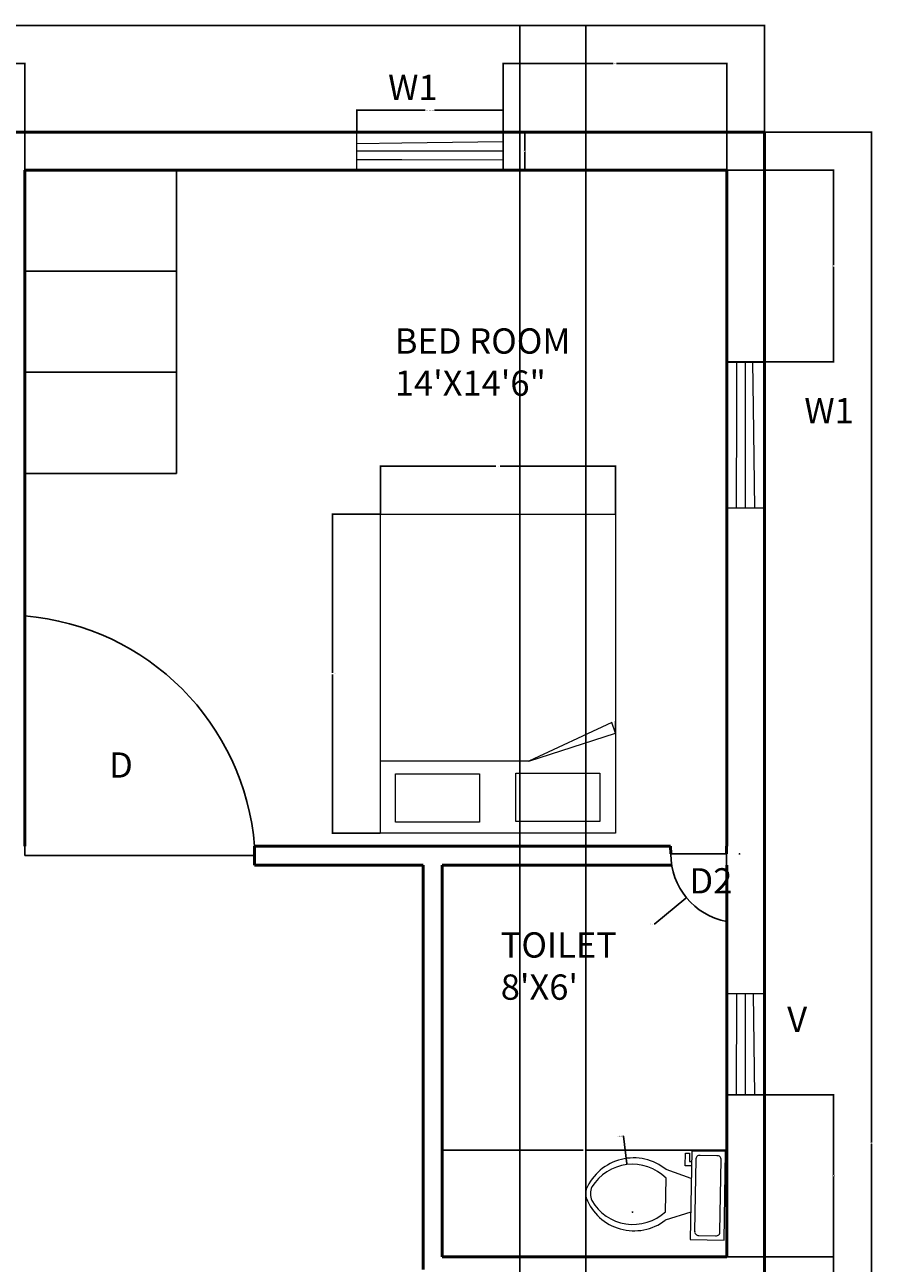
# Model space of a CAD drawing. Units: inches. Extents: x 2521 to 2933, y 1745 to 2276.
# Tile 4 of 4: x 2731 to 2933, y 1982 to 2276. Entities that reach past the tile are written whole.
import ezdxf

# ---------------------------------------------------------------- set-up
doc = ezdxf.new("R2010")
doc.units = ezdxf.units.IN
for name, color, linetype, lineweight in [('A-ANNO-DIMS', 2, 'Continuous', 18), ('A-ANNO-TEXT', 3, 'Continuous', 18), ('A-AREA-IDEN', 7, 'Continuous', 25), ('A-DOOR', 3, 'Continuous', 25), ('A-FLOR-CASE', 32, 'Continuous', 25), ('A-FLOR-FIXT', 9, 'Continuous', 18), ('A-FURN', 8, 'Continuous', 18), ('A-GLAZ', 4, 'Continuous', 20), ('A-WALL', 7, 'Continuous', 50)]:
    doc.layers.add(name, color=color, linetype=linetype, lineweight=lineweight)
doc.styles.get("Standard").update_dxf_attribs({"font": 'arial.ttf'})
doc.dimstyles.get("Standard").update_dxf_attribs({"dimtxt": 0.18, "dimasz": 0.18, "dimexe": 0.18, "dimexo": 0.0625, "dimgap": 0.09, "dimtad": 0, "dimtih": 1, "dimtoh": 1, "dimdec": 4, "dimzin": 0, "dimdsep": 46, "dimtxsty": 'Standard', "dimcen": 0.09, "dimadec": 0, "dimazin": 0, "dimtfac": 1, "dimtdec": 4, "dimtofl": 0, "dimtmove": 0, "dimatfit": 3, "dimfxl": 1, "dimtolj": 1, "dimtzin": 0, "dimarcsym": 0})

# ---------------------------------------------------------------- blocks, each defined once
blk = doc.blocks.new('Toilet - top')
for p, q in [((9.5, -6), (9.5, -2)), ((-10, -8.5), (-8, -8.5)), ((-10, -9.5), (-10, -8.5)), ((-8, -8.5), (-8, -8)), ((-7, -8), (-7, -9.5)), ((-4, -8), (-6, -14)), ((4, -8), (6, -14)), ((-7, -9.5), (-10, -9.5)), ((4, -14), (-4, -14))]:
    blk.add_line(p, q)
blk.add_lwpolyline([(10.5, -8), (10.5, 0), (-10.5, 0), (-10.5, -8)], close=True)
for points in [[(-9.5, -2), (-9.5, -6)], [(8.5, -1), (-8.5, -1)], [(-8.5, -7), (8.5, -7)]]:
    blk.add_lwpolyline(points)
for centre, radius, start, end in [((-8.62, -1.88), 0.884, 81.8699, 188.1301), ((8.62, -1.88), 0.884, 351.8699, 98.1301), ((-8.62, -6.12), 0.884, 171.8699, 278.1301), ((8.62, -6.12), 0.884, 261.8699, 8.1301), ((3.52, -21.58), 12.17, 141.4691, 247.9714), ((4.2, -21.82), 11.33, 136.3677, 238.9468), ((-3.52, -21.58), 12.17, 292.0284, 38.5307), ((-4.2, -21.82), 11.33, 301.053, 43.6321), ((0, -27.88), 4, 245.7318, 294.2682), ((0, -29), 4, 254.8605, 285.1395)]:
    blk.add_arc(centre, radius, start, end)
blk = doc.blocks.new('WINDOW-W1-LONG')
for p, q in [((0, 24), (0, 34.69)), ((0, 34.69), (9, 34.69)), ((2.4, 24), (2.44, 34.69)), ((4.5, 24), (4.5, 34.69)), ((6.37, 24), (6.23, 34.69)), ((9, 34.69), (9, 24)), ((0, 24), (0, 0)), ((2.32, 0), (2.4, 24)), ((4.5, 0), (4.5, 24)), ((6.68, 0), (6.37, 24)), ((9, 24), (9, 0)), ((9, 0), (0, 0))]:
    blk.add_line(p, q)
blk = doc.blocks.new('WINDOW-24')
for p, q in [((9, 24), (0, 24)), ((0, 24), (0, 0)), ((2.32, 0), (2.4, 24)), ((4.5, 0), (4.5, 24)), ((6.68, 0), (6.37, 24)), ((9, 24), (9, 0)), ((9, 0), (0, 0))]:
    blk.add_line(p, q)
blk = doc.blocks.new('DOOR-SINGLE-SWING')
for p, q in [((54.54, 0), (54.54, 56.86)), ((0, 0), (54.54, 0))]:
    blk.add_line(p, q)
blk.add_arc((59.46, -2.59), 59.65, 94.7338, 175.398)
blk = doc.blocks.new('BED-DOUBLE')
for p, q in [((55.72, 23.76), (55.72, 26.62)), ((54.9, 26.24), (35.19, 17.12)), ((35.19, 17.12), (55.72, 23.76)), ((55.72, 23.76), (54.9, 26.24)), ((35.19, 17.12), (0, 17.12))]:
    blk.add_line(p, q)
for points in [[(0, 75.73), (55.72, 75.73), (55.72, 0), (0, 0)], [(3.53, 14.11), (23.44, 14.11), (23.44, 2.6), (3.53, 2.6)], [(32.11, 14.25), (52.02, 14.25), (52.02, 2.74), (32.11, 2.74)]]:
    blk.add_lwpolyline(points, close=True)
blk = doc.blocks.new('CABINET-3-BAY')
for p, q in [((0, 0), (0, 72)), ((0, 48), (36, 48)), ((0, 24), (36, 24)), ((0, 0), (36, 0))]:
    blk.add_line(p, q)
blk = doc.blocks.new('*D9')
at = {"layer": 'A-ANNO-DIMS', "color": 0, "lineweight": -2, "transparency": 16777216}
for p, q in [((2810.24, 2250.34), (2810.24, 2255.67)), ((2810.42, 2255.49), (2826.47, 2255.49)), ((2844.76, 2255.49), (2828.71, 2255.49)), ((2844.94, 2250.34), (2844.94, 2255.67))]:
    blk.add_line(p, q, dxfattribs=at)
at = {"layer": 'A-ANNO-DIMS', "color": 0, "transparency": 16777216}
for points in [[(2810.42, 2255.52), (2810.42, 2255.46), (2810.24, 2255.49)], [(2844.76, 2255.52), (2844.76, 2255.46), (2844.94, 2255.49)]]:
    blk.add_solid(points, dxfattribs=at)
at = {"layer": 'Defpoints', "color": 0, "transparency": 16777216}
for p in [(2810.24, 2255.49), (2810.24, 2250.28), (2844.94, 2250.28)]:
    blk.add_point(p, dxfattribs=at)
at = {"layer": 'A-ANNO-DIMS', "color": 0, "transparency": 16777216, "insert": (2827.59, 2255.49), "char_height": 0.18, "attachment_point": 5}
blk.add_mtext('\\A1;WINDOW 35 TYP.', dxfattribs=at)
blk = doc.blocks.new('*D10')
at = {"layer": 'A-ANNO-DIMS', "color": 0, "lineweight": -2, "transparency": 16777216}
for p, q in [((2845, 2250.28), (2850.32, 2250.28)), ((2850.14, 2250.1), (2850.14, 2245.96)), ((2850.14, 2241.46), (2850.14, 2245.6)), ((2845, 2241.28), (2850.32, 2241.28))]:
    blk.add_line(p, q, dxfattribs=at)
at = {"layer": 'A-ANNO-DIMS', "color": 0, "transparency": 16777216}
for points in [[(2850.11, 2250.1), (2850.17, 2250.1), (2850.14, 2250.28)], [(2850.11, 2241.46), (2850.17, 2241.46), (2850.14, 2241.28)]]:
    blk.add_solid(points, dxfattribs=at)
at = {"layer": 'Defpoints', "color": 0, "transparency": 16777216}
for p in [(2844.94, 2250.28), (2850.14, 2250.28), (2844.94, 2241.28)]:
    blk.add_point(p, dxfattribs=at)
at = {"layer": 'A-ANNO-DIMS', "color": 0, "transparency": 16777216, "insert": (2850.14, 2245.78), "char_height": 0.18, "attachment_point": 5}
blk.add_mtext('\\A1;9 TYP.', dxfattribs=at)
blk = doc.blocks.new('*D13')
at = {"layer": 'A-ANNO-DIMS', "color": 0, "lineweight": -2, "transparency": 16777216}
for p, q in [((2815.82, 2159.61), (2804.34, 2159.61)), ((2804.52, 2159.43), (2804.52, 2121.93)), ((2804.52, 2084.06), (2804.52, 2121.56)), ((2815.82, 2083.88), (2804.34, 2083.88))]:
    blk.add_line(p, q, dxfattribs=at)
at = {"layer": 'A-ANNO-DIMS', "color": 0, "transparency": 16777216}
for points in [[(2804.49, 2159.43), (2804.55, 2159.43), (2804.52, 2159.61)], [(2804.49, 2084.06), (2804.55, 2084.06), (2804.52, 2083.88)]]:
    blk.add_solid(points, dxfattribs=at)
at = {"layer": 'Defpoints', "color": 0, "transparency": 16777216}
for p in [(2804.52, 2159.61), (2815.88, 2159.61), (2815.88, 2083.88)]:
    blk.add_point(p, dxfattribs=at)
at = {"layer": 'A-ANNO-DIMS', "color": 0, "transparency": 16777216, "insert": (2804.52, 2121.74), "char_height": 0.18, "attachment_point": 5}
blk.add_mtext('\\A1;BED 76 TYP.', dxfattribs=at)
blk = doc.blocks.new('*D14')
at = {"layer": 'A-ANNO-DIMS', "color": 0, "lineweight": -2, "transparency": 16777216}
for p, q in [((2815.88, 2159.67), (2815.88, 2171.15)), ((2816.06, 2170.97), (2843.21, 2170.97)), ((2871.42, 2170.97), (2844.27, 2170.97)), ((2871.6, 2159.67), (2871.6, 2171.15))]:
    blk.add_line(p, q, dxfattribs=at)
at = {"layer": 'A-ANNO-DIMS', "color": 0, "transparency": 16777216}
for points in [[(2816.06, 2171), (2816.06, 2170.94), (2815.88, 2170.97)], [(2871.42, 2171), (2871.42, 2170.94), (2871.6, 2170.97)]]:
    blk.add_solid(points, dxfattribs=at)
at = {"layer": 'Defpoints', "color": 0, "transparency": 16777216}
for p in [(2871.6, 2170.97), (2815.88, 2159.61), (2871.6, 2159.61)]:
    blk.add_point(p, dxfattribs=at)
at = {"layer": 'A-ANNO-DIMS', "color": 0, "transparency": 16777216, "insert": (2843.74, 2170.97), "char_height": 0.18, "attachment_point": 5}
blk.add_mtext('\\A1;56 TYP.', dxfattribs=at)
blk = doc.blocks.new('*D23')
at = {"layer": 'A-ANNO-DIMS', "color": 0, "lineweight": -2, "transparency": 16777216}
for p, q in [((2547.01, 2250.34), (2547.01, 2275.78)), ((2547.19, 2275.6), (2726.72, 2275.6)), ((2906.83, 2275.6), (2727.3, 2275.6)), ((2907.01, 2250.34), (2907.01, 2275.78))]:
    blk.add_line(p, q, dxfattribs=at)
at = {"layer": 'A-ANNO-DIMS', "color": 0, "transparency": 16777216}
for points in [[(2547.19, 2275.63), (2547.19, 2275.57), (2547.01, 2275.6)], [(2906.83, 2275.63), (2906.83, 2275.57), (2907.01, 2275.6)]]:
    blk.add_solid(points, dxfattribs=at)
at = {"layer": 'Defpoints', "color": 0, "transparency": 16777216}
for p in [(2907.01, 2275.6), (2547.01, 2250.28), (2907.01, 2250.28)]:
    blk.add_point(p, dxfattribs=at)
at = {"layer": 'A-ANNO-DIMS', "color": 0, "transparency": 16777216, "insert": (2727.01, 2275.6), "char_height": 0.18, "attachment_point": 5}
blk.add_mtext('\\A1;360', dxfattribs=at)
blk = doc.blocks.new('*D24')
at = {"layer": 'A-ANNO-DIMS', "color": 0, "lineweight": -2, "transparency": 16777216}
for p, q in [((2907.07, 2250.28), (2932.51, 2250.28)), ((2932.33, 2250.1), (2932.33, 2010.46)), ((2932.33, 1770.46), (2932.33, 2010.1)), ((2907.07, 1770.28), (2932.51, 1770.28))]:
    blk.add_line(p, q, dxfattribs=at)
at = {"layer": 'A-ANNO-DIMS', "color": 0, "transparency": 16777216}
for points in [[(2932.3, 2250.1), (2932.36, 2250.1), (2932.33, 2250.28)], [(2932.3, 1770.46), (2932.36, 1770.46), (2932.33, 1770.28)]]:
    blk.add_solid(points, dxfattribs=at)
at = {"layer": 'Defpoints', "color": 0, "transparency": 16777216}
for p in [(2907.01, 2250.28), (2932.33, 2250.28), (2907.01, 1770.28)]:
    blk.add_point(p, dxfattribs=at)
at = {"layer": 'A-ANNO-DIMS', "color": 0, "transparency": 16777216, "insert": (2932.33, 2010.28), "char_height": 0.18, "attachment_point": 5}
blk.add_mtext('\\A1;480', dxfattribs=at)
blk = doc.blocks.new('*D27')
at = {"layer": 'A-ANNO-DIMS', "color": 0, "lineweight": -2, "transparency": 16777216}
for p, q in [((2722.51, 2241.34), (2722.51, 2266.78)), ((2731.51, 2241.34), (2731.51, 2266.78)), ((2722.69, 2266.6), (2726.86, 2266.6)), ((2731.33, 2266.6), (2727.16, 2266.6))]:
    blk.add_line(p, q, dxfattribs=at)
at = {"layer": 'A-ANNO-DIMS', "color": 0, "transparency": 16777216}
for points in [[(2722.69, 2266.63), (2722.69, 2266.57), (2722.51, 2266.6)], [(2731.33, 2266.63), (2731.33, 2266.57), (2731.51, 2266.6)]]:
    blk.add_solid(points, dxfattribs=at)
at = {"layer": 'Defpoints', "color": 0, "transparency": 16777216}
for p in [(2731.51, 2266.6), (2722.51, 2241.28), (2731.51, 2241.28)]:
    blk.add_point(p, dxfattribs=at)
at = {"layer": 'A-ANNO-DIMS', "color": 0, "transparency": 16777216, "insert": (2727.01, 2266.6), "char_height": 0.18, "attachment_point": 5}
blk.add_mtext('\\A1;9', dxfattribs=at)
blk = doc.blocks.new('*D28')
at = {"layer": 'A-ANNO-DIMS', "color": 0, "lineweight": -2, "transparency": 16777216}
for p, q in [((2844.94, 2241.34), (2844.94, 2266.78)), ((2898.01, 2241.34), (2898.01, 2266.78)), ((2845.12, 2266.6), (2871.08, 2266.6)), ((2897.83, 2266.6), (2871.87, 2266.6))]:
    blk.add_line(p, q, dxfattribs=at)
at = {"layer": 'A-ANNO-DIMS', "color": 0, "transparency": 16777216}
for points in [[(2845.12, 2266.63), (2845.12, 2266.57), (2844.94, 2266.6)], [(2897.83, 2266.63), (2897.83, 2266.57), (2898.01, 2266.6)]]:
    blk.add_solid(points, dxfattribs=at)
at = {"layer": 'Defpoints', "color": 0, "transparency": 16777216}
for p in [(2898.01, 2266.6), (2844.94, 2241.28), (2898.01, 2241.28)]:
    blk.add_point(p, dxfattribs=at)
at = {"layer": 'A-ANNO-DIMS', "color": 0, "transparency": 16777216, "insert": (2871.47, 2266.6), "char_height": 0.18, "attachment_point": 5}
blk.add_mtext('\\A1;53.07', dxfattribs=at)
blk = doc.blocks.new('*D36')
at = {"layer": 'A-ANNO-DIMS', "color": 0, "lineweight": -2, "transparency": 16777216}
for p, q in [((2898.07, 1983.28), (2923.51, 1983.28)), ((2923.33, 1983.1), (2923.33, 1960.51)), ((2923.33, 1937.55), (2923.33, 1960.14)), ((2898.07, 1937.37), (2923.51, 1937.37))]:
    blk.add_line(p, q, dxfattribs=at)
at = {"layer": 'A-ANNO-DIMS', "color": 0, "transparency": 16777216}
for points in [[(2923.3, 1983.1), (2923.36, 1983.1), (2923.33, 1983.28)], [(2923.3, 1937.55), (2923.36, 1937.55), (2923.33, 1937.37)]]:
    blk.add_solid(points, dxfattribs=at)
at = {"layer": 'Defpoints', "color": 0, "transparency": 16777216}
for p in [(2898.01, 1983.28), (2898.01, 1937.37), (2923.33, 1937.37)]:
    blk.add_point(p, dxfattribs=at)
at = {"layer": 'A-ANNO-DIMS', "color": 0, "transparency": 16777216, "insert": (2923.33, 1960.32), "char_height": 0.18, "attachment_point": 5}
blk.add_mtext('\\A1;45.91', dxfattribs=at)
blk = doc.blocks.new('*D37')
at = {"layer": 'A-ANNO-DIMS', "color": 0, "lineweight": -2, "transparency": 16777216}
for p, q in [((2898.07, 2021.77), (2923.51, 2021.77)), ((2923.33, 2021.59), (2923.33, 2002.71)), ((2923.33, 1983.46), (2923.33, 2002.34)), ((2898.07, 1983.28), (2923.51, 1983.28))]:
    blk.add_line(p, q, dxfattribs=at)
at = {"layer": 'A-ANNO-DIMS', "color": 0, "transparency": 16777216}
for points in [[(2923.3, 2021.59), (2923.36, 2021.59), (2923.33, 2021.77)], [(2923.3, 1983.46), (2923.36, 1983.46), (2923.33, 1983.28)]]:
    blk.add_solid(points, dxfattribs=at)
at = {"layer": 'Defpoints', "color": 0, "transparency": 16777216}
for p in [(2898.01, 2021.77), (2898.01, 1983.28), (2923.33, 1983.28)]:
    blk.add_point(p, dxfattribs=at)
at = {"layer": 'A-ANNO-DIMS', "color": 0, "transparency": 16777216, "insert": (2923.33, 2002.52), "char_height": 0.18, "attachment_point": 5}
blk.add_mtext('\\A1;38.485', dxfattribs=at)
blk = doc.blocks.new('*D38')
at = {"layer": 'A-ANNO-DIMS', "color": 0, "lineweight": -2, "transparency": 16777216}
for p, q in [((2898.07, 2241.28), (2923.51, 2241.28)), ((2923.33, 2241.1), (2923.33, 2218.69)), ((2923.33, 2195.91), (2923.33, 2218.32)), ((2898.07, 2195.73), (2923.51, 2195.73))]:
    blk.add_line(p, q, dxfattribs=at)
at = {"layer": 'A-ANNO-DIMS', "color": 0, "transparency": 16777216}
for points in [[(2923.3, 2241.1), (2923.36, 2241.1), (2923.33, 2241.28)], [(2923.3, 2195.91), (2923.36, 2195.91), (2923.33, 2195.73)]]:
    blk.add_solid(points, dxfattribs=at)
at = {"layer": 'Defpoints', "color": 0, "transparency": 16777216}
for p in [(2898.01, 2241.28), (2898.01, 2195.73), (2923.33, 2195.73)]:
    blk.add_point(p, dxfattribs=at)
at = {"layer": 'A-ANNO-DIMS', "color": 0, "transparency": 16777216, "insert": (2923.33, 2218.5), "char_height": 0.18, "attachment_point": 5}
blk.add_mtext('\\A1;45.56', dxfattribs=at)
blk = doc.blocks.new('*D49')
at = {"layer": 'A-ANNO-DIMS', "color": 0, "lineweight": -2, "transparency": 16777216}
for p, q in [((2830.51, 1983.34), (2830.51, 2008.78)), ((2830.69, 2008.6), (2863.93, 2008.6)), ((2897.83, 2008.6), (2864.58, 2008.6)), ((2898.01, 1983.34), (2898.01, 2008.78))]:
    blk.add_line(p, q, dxfattribs=at)
at = {"layer": 'A-ANNO-DIMS', "color": 0, "transparency": 16777216}
for points in [[(2830.69, 2008.63), (2830.69, 2008.57), (2830.51, 2008.6)], [(2897.83, 2008.63), (2897.83, 2008.57), (2898.01, 2008.6)]]:
    blk.add_solid(points, dxfattribs=at)
at = {"layer": 'Defpoints', "color": 0, "transparency": 16777216}
for p in [(2898.01, 2008.6), (2830.51, 1983.28), (2898.01, 1983.28)]:
    blk.add_point(p, dxfattribs=at)
at = {"layer": 'A-ANNO-DIMS', "color": 0, "transparency": 16777216, "insert": (2864.26, 2008.6), "char_height": 0.18, "attachment_point": 5}
blk.add_mtext('\\A1;67.5', dxfattribs=at)
blk = doc.blocks.new('*D59')
at = {"layer": 'A-ANNO-DIMS', "color": 0, "lineweight": -2, "transparency": 16777216}
for p, q in [((2848.92, 1927.91), (2848.92, 2275.78)), ((2849.1, 2275.6), (2856.29, 2275.6)), ((2864.39, 2275.6), (2857.2, 2275.6)), ((2864.57, 1950.23), (2864.57, 2275.78))]:
    blk.add_line(p, q, dxfattribs=at)
at = {"layer": 'A-ANNO-DIMS', "color": 0, "transparency": 16777216}
for points in [[(2849.1, 2275.63), (2849.1, 2275.57), (2848.92, 2275.6)], [(2864.39, 2275.63), (2864.39, 2275.57), (2864.57, 2275.6)]]:
    blk.add_solid(points, dxfattribs=at)
at = {"layer": 'Defpoints', "color": 0, "transparency": 16777216}
for p in [(2864.57, 2275.6), (2864.57, 1950.17), (2848.92, 1927.85)]:
    blk.add_point(p, dxfattribs=at)
at = {"layer": 'A-ANNO-DIMS', "color": 0, "transparency": 16777216, "insert": (2856.74, 2275.6), "char_height": 0.18, "attachment_point": 5}
blk.add_mtext('\\A1;15.656', dxfattribs=at)
blk = doc.blocks.new('*D62')
at = {"layer": 'A-ANNO-DIMS', "color": 0, "lineweight": -2, "transparency": 16777216}
for p, q in [((2900.94, 2078.93), (2901.12, 2078.93)), ((2901.03, 2078.84), (2901.03, 2079.02)), ((2880.95, 2062.32), (2888.35, 2068.43)), ((2880.77, 2062.32), (2880.95, 2062.32))]:
    blk.add_line(p, q, dxfattribs=at)
at = {"layer": 'A-ANNO-DIMS', "color": 0, "transparency": 16777216}
blk.add_solid([(2888.33, 2068.45), (2888.36, 2068.41), (2888.48, 2068.55)], dxfattribs=at)
at = {"layer": 'Defpoints', "color": 0, "transparency": 16777216}
for p in [(2901.03, 2078.93), (2888.48, 2068.55)]:
    blk.add_point(p, dxfattribs=at)
at = {"layer": 'A-ANNO-DIMS', "color": 0, "transparency": 16777216, "insert": (2880.23, 2062.32), "char_height": 0.18, "attachment_point": 5}
blk.add_mtext('\\A1;R16.286', dxfattribs=at)
blk = doc.blocks.new('*D65')
at = {"layer": 'A-ANNO-DIMS', "color": 0, "lineweight": -2, "transparency": 16777216}
for p, q in [((2873.36, 2011.94), (2873.54, 2011.94)), ((2873.54, 2011.94), (2874.32, 2005.37)), ((2875.57, 1993.94), (2875.75, 1993.94)), ((2875.66, 1993.85), (2875.66, 1994.03))]:
    blk.add_line(p, q, dxfattribs=at)
at = {"layer": 'A-ANNO-DIMS', "color": 0, "transparency": 16777216}
blk.add_solid([(2874.35, 2005.37), (2874.29, 2005.36), (2874.34, 2005.19)], dxfattribs=at)
at = {"layer": 'Defpoints', "color": 0, "transparency": 16777216}
for p in [(2874.34, 2005.19), (2875.66, 1993.94)]:
    blk.add_point(p, dxfattribs=at)
at = {"layer": 'A-ANNO-DIMS', "color": 0, "transparency": 16777216, "insert": (2872.69, 2011.94), "char_height": 0.18, "attachment_point": 5}
blk.add_mtext('\\A1;4X R11.33', dxfattribs=at)

msp = doc.modelspace()

# ---------------------------------------------------------------- linework, layer by layer
at = {"layer": 'A-DOOR'}
for p, q in [((2884.7464, 2078.9456), (2898.0014, 2078.9456)), ((2898.0014, 2078.9456), (2898.0014, 2062.9248))]:
    msp.add_line(p, q, dxfattribs=at)
msp.add_arc((2901.0328, 2078.9266), 16.2864, 179.93294, 259.273035, dxfattribs=at)
at = {"layer": 'A-WALL'}
for p, q in [((2547.009, 2250.2819), (2907.009, 2250.2819)), ((2907.009, 2250.2819), (2907.009, 1770.2819)), ((2731.509, 2080.7819), (2731.509, 2241.2819)), ((2731.509, 2241.2819), (2898.009, 2241.2819)), ((2898.009, 2241.2819), (2898.009, 2080.7819)), ((2786.0146, 2080.7819), (2786.0146, 2078.585)), ((2884.7023, 2080.7819), (2786.0146, 2080.7819)), ((2786.0146, 2078.585), (2786.0146, 2076.2819)), ((2884.7464, 2078.9456), (2884.7023, 2080.7819)), ((2898.009, 2080.7819), (2898.0014, 2080.7819)), ((2898.0014, 2078.9456), (2898.0014, 2080.7819)), ((2786.0146, 2076.2819), (2826.009, 2076.2819)), ((2826.009, 1980.2819), (2826.009, 2076.2819)), ((2830.509, 1983.2819), (2830.509, 2076.2819)), ((2884.9625, 2076.2819), (2830.509, 2076.2819)), ((2898.009, 2076.2819), (2898.0014, 2076.2819)), ((2898.009, 2076.2819), (2898.009, 1983.2819)), ((2830.509, 1983.2819), (2898.009, 1983.2819))]:
    msp.add_line(p, q, dxfattribs=at)

# ---------------------------------------------------------------- block references
at = {"layer": 'A-DOOR', "extrusion": (0, 0, -1), "zscale": -1}
msp.add_blockref('DOOR-SINGLE-SWING', (-2786.0151, 2078.585), dxfattribs=at)
at = {"layer": 'A-FLOR-CASE', "extrusion": (0, 0, -1), "zscale": -1}
msp.add_blockref('CABINET-3-BAY', (-2767.5091, 2169.282), dxfattribs=at)
at = {"layer": 'A-FLOR-FIXT', "rotation": 269.0579063208954}
msp.add_blockref('Toilet - top', (2897.5453, 1997.7762), dxfattribs=at)
at = {"layer": 'A-FURN'}
msp.add_blockref('BED-DOUBLE', (2815.8826, 2083.8816), dxfattribs=at)
at = {"layer": 'A-GLAZ', "rotation": 89.99999999999766}
msp.add_blockref('WINDOW-W1-LONG', (2844.9366, 2241.2819), dxfattribs=at)
at = {"layer": 'A-GLAZ'}
for name, p in [('WINDOW-W1-LONG', (2898.009, 2161.0317)), ('WINDOW-24', (2898.009, 2021.7669))]:
    msp.add_blockref(name, p, dxfattribs=at)

# ---------------------------------------------------------------- texts
at = {"layer": 'A-ANNO-TEXT', "char_height": 6, "attachment_point": 1}
for s, width, insert in [('W1', 10.814281, (2817.6837, 2263.9193)), ('W1', 10.559342, (2916.4285, 2187.1685)), ('D', 11.775491, (2751.4953, 2103.0512)), ('D2', 4.490782, (2889.1703, 2075.5606)), ('V', 11.777725, (2912.3704, 2042.6568))]:
    msp.add_mtext_dynamic_manual_height_columns(s, width=width, gutter_width=5.8967, heights=[0], dxfattribs=dict(at, insert=insert))
at = {"layer": 'A-AREA-IDEN', "char_height": 6, "attachment_point": 1}
for s, width, insert in [('BED ROOM \\P14\'X14\'6"', 50.277821, (2819.2707, 2203.7086)), ("TOILET\\P8'X6'", 38.619361, (2844.4003, 2060.3331))]:
    msp.add_mtext_dynamic_manual_height_columns(s, width=width, gutter_width=5.8967, heights=[0], dxfattribs=dict(at, insert=insert))

# ---------------------------------------------------------------- dimensions: what is measured, and where the dimension line sits
at = {"layer": 'A-ANNO-DIMS'}
for base, p1, p2, override, picture, middle in [((2907.009, 2275.6019), (2547.009, 2250.2819), (2907.009, 2250.2819), {"dimdec": 0, "dimlfac": 1, "dimrnd": 0, "dimzin": 0, "dimdsep": 46, "dimlunit": 2}, '*D23', (2727.009, 2275.6019)), ((2864.5724, 2275.6019), (2848.9165, 1927.8472), (2864.5724, 1950.1723), {"dimdec": 3, "dimlfac": 1, "dimrnd": 0, "dimzin": 0, "dimdsep": 46, "dimlunit": 2}, '*D59', (2856.7445, 2275.6019)), ((2731.509, 2266.6019), (2722.509, 2241.2819), (2731.509, 2241.2819), {"dimdec": 0, "dimlfac": 1, "dimrnd": 0, "dimzin": 0, "dimdsep": 46, "dimlunit": 2}, '*D27', (2727.009, 2266.6019)), ((2898.009, 2266.6019), (2844.9364, 2241.2819), (2898.009, 2241.2819), {"dimdec": 2, "dimlfac": 1, "dimrnd": 0, "dimzin": 0, "dimdsep": 46, "dimlunit": 2}, '*D28', (2871.4727, 2266.6019)), ((2898.009, 2008.6019), (2830.509, 1983.2819), (2898.009, 1983.2819), {"dimdec": 1, "dimlfac": 1, "dimrnd": 0, "dimzin": 0, "dimdsep": 46, "dimlunit": 2}, '*D49', (2864.259, 2008.6019))]:
    dim = msp.add_linear_dim(base=base, p1=p1, p2=p2, dimstyle='Standard', override=override, dxfattribs=at)
    dim.commit()
    dim.dimension.update_dxf_attribs({"geometry": picture, "text_midpoint": middle})
for base, p1, p2, angle, text, picture, middle in [((2810.2421, 2255.486), (2844.9364, 2250.2819), (2810.2421, 2250.2819), 180, 'WINDOW <> TYP.', '*D9', (2827.5892, 2255.486)), ((2850.1405, 2250.2819), (2844.9364, 2241.2819), (2844.9364, 2250.2819), 90, '<> TYP.', '*D10', (2850.1405, 2245.7819)), ((2804.5236, 2159.608), (2815.8825, 2083.8819), (2815.8825, 2159.608), 90, 'BED <> TYP.', '*D13', (2804.5236, 2121.7449))]:
    dim = msp.add_linear_dim(base=base, p1=p1, p2=p2, angle=angle, text=text, dimstyle='Standard', override={"dimdec": 0, "dimlfac": 1, "dimrnd": 0, "dimzin": 0, "dimdsep": 46, "dimlunit": 2}, dxfattribs=at)
    dim.commit()
    dim.dimension.update_dxf_attribs({"geometry": picture, "text_midpoint": middle})
for base, p1, p2, angle, override, picture, middle in [((2932.329, 2250.2819), (2907.009, 1770.2819), (2907.009, 2250.2819), 90, {"dimdec": 0, "dimlfac": 1, "dimrnd": 0, "dimzin": 0, "dimdsep": 46, "dimlunit": 2}, '*D24', (2932.329, 2010.2819)), ((2923.329, 2195.7261), (2898.009, 2241.2819), (2898.009, 2195.7261), 270, {"dimdec": 2, "dimlfac": 1, "dimrnd": 0, "dimzin": 0, "dimdsep": 46, "dimlunit": 2}, '*D38', (2923.329, 2218.504)), ((2923.329, 1983.2819), (2898.009, 2021.7666), (2898.009, 1983.2819), 270, {"dimdec": 3, "dimlfac": 1, "dimrnd": 0, "dimzin": 0, "dimdsep": 46, "dimlunit": 2}, '*D37', (2923.329, 2002.5243)), ((2923.329, 1937.3677), (2898.009, 1983.2819), (2898.009, 1937.3677), 270, {"dimdec": 2, "dimlfac": 1, "dimrnd": 0, "dimzin": 0, "dimdsep": 46, "dimlunit": 2}, '*D36', (2923.329, 1960.3248))]:
    dim = msp.add_linear_dim(base=base, p1=p1, p2=p2, angle=angle, dimstyle='Standard', override=override, dxfattribs=at)
    dim.commit()
    dim.dimension.update_dxf_attribs({"geometry": picture, "text_midpoint": middle})
dim = msp.add_linear_dim(base=(2871.6013, 2170.9669), p1=(2815.8825, 2159.608), p2=(2871.6013, 2159.608), text='<> TYP.', dimstyle='Standard', override={"dimdec": 0, "dimlfac": 1, "dimrnd": 0, "dimzin": 0, "dimdsep": 46, "dimlunit": 2}, dxfattribs=at)
dim.commit()
dim.dimension.update_dxf_attribs({"geometry": '*D14', "text_midpoint": (2843.7419, 2170.9669)})
dim = msp.add_radius_dim(center=(2901.0328, 2078.9266), mpoint=(2888.4841, 2068.545), dimstyle='Standard', override={"dimdec": 3, "dimlfac": 1, "dimrnd": 0, "dimzin": 0, "dimdsep": 46, "dimlunit": 2}, dxfattribs=at)
dim.commit()
dim.dimension.update_dxf_attribs({"geometry": '*D62', "text_midpoint": (2880.2251, 2062.3161), "dimtype": 164})
dim = msp.add_radius_dim(center=(2875.6618, 1993.9356), mpoint=(2874.337, 2005.187), text='4X <>', dimstyle='Standard', override={"dimdec": 2, "dimlfac": 1, "dimrnd": 0, "dimzin": 0, "dimdsep": 46, "dimlunit": 2}, dxfattribs=at)
dim.commit()
dim.dimension.update_dxf_attribs({"geometry": '*D65', "text_midpoint": (2872.6853, 2011.9379), "dimtype": 164})

doc.saveas('drawing.dxf')
